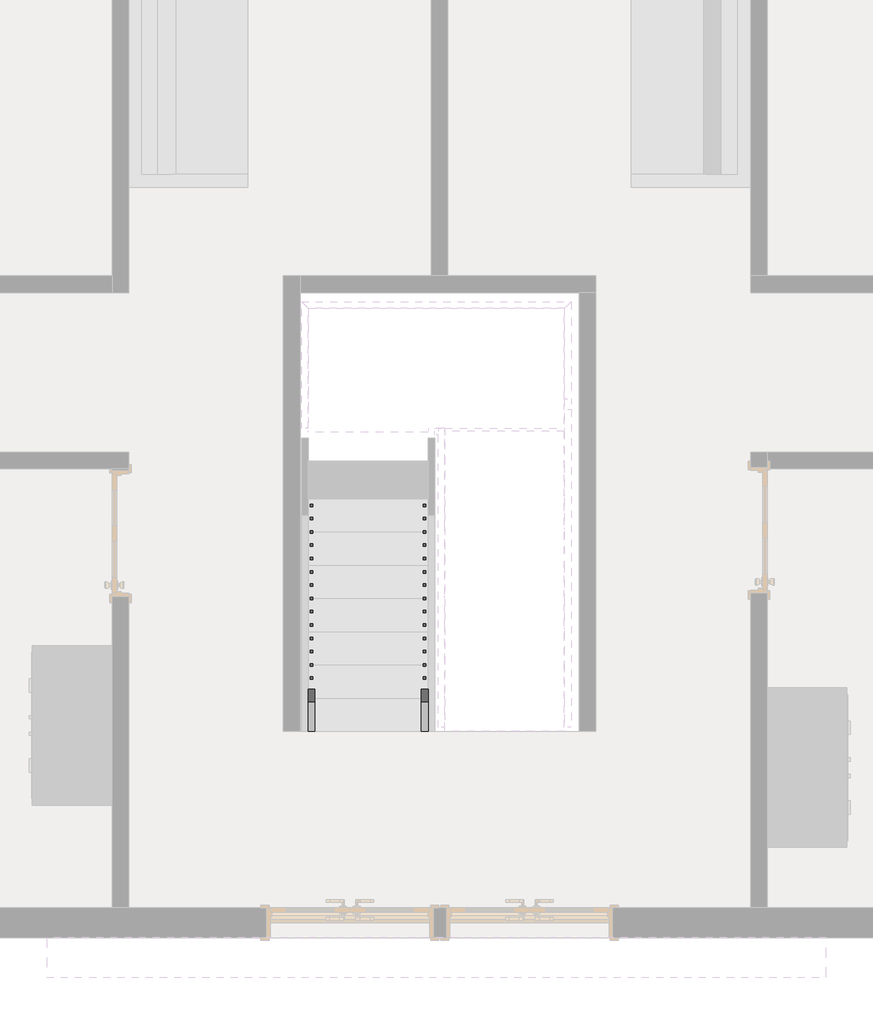
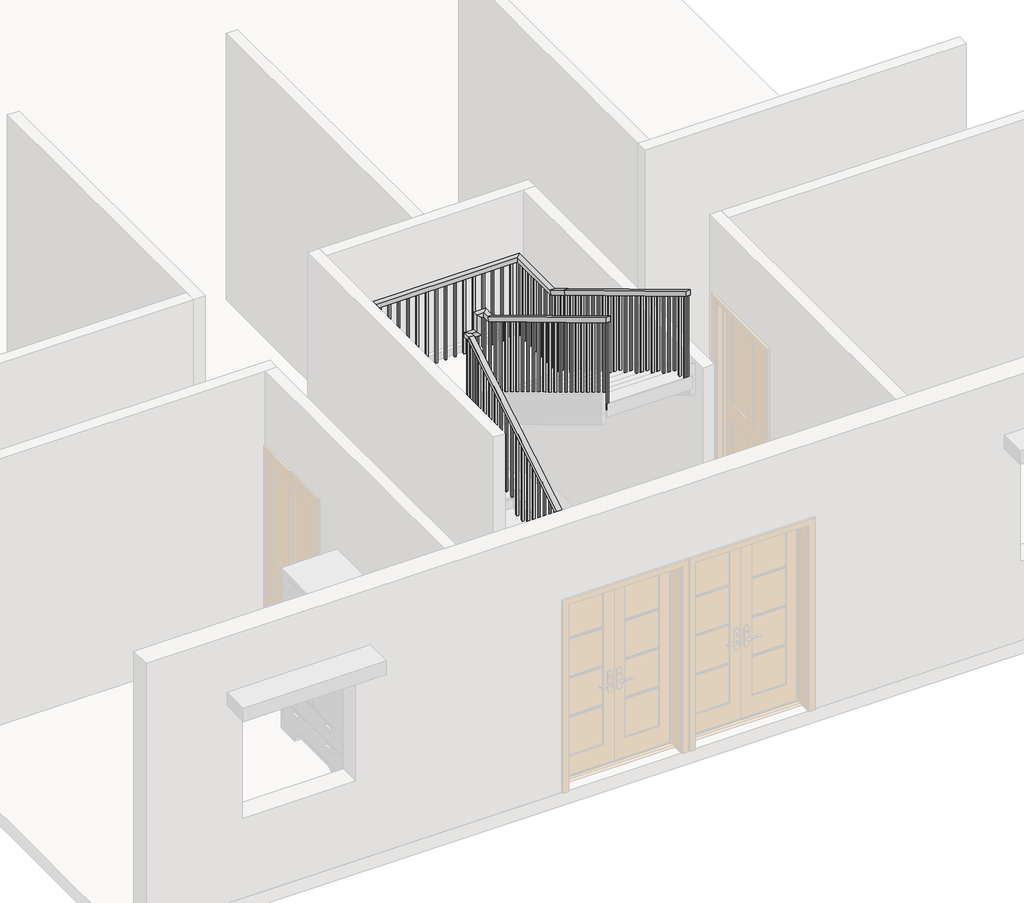
# One storey, part 3 of 4: 2 railings.
"""IFC4 building model written with IfcOpenShell, lengths in millimetres."""

from ifc_helpers import new_model, si_unit, frame, origin, place, context, project, spatial, polyline, outline, extrude, faceted_brep, element, save

model = new_model("IFC4")

# Units and contexts
model_context = context("Model", 3, world=origin())
ifc_project = project(units=[si_unit("LENGTHUNIT", "METRE", prefix="MILLI")], contexts=[model_context])

# Site, building, storey
site = spatial("IfcSite", under=ifc_project)
building = spatial("IfcBuilding", under=site)
storey = spatial("IfcBuildingStorey", under=building, Elevation=0.0)

# Railings
placement = place(None, origin())
element("IfcRailing", 1, ObjectType="Handrail - Rectangular", at=placement, inside=storey, context=model_context, shape_type="SolidModel", body=[
    faceted_brep([(-9678.6771954, -4957.4727897, 1066.8), (-9678.6771954, -4957.4727897, 1007.5575287), (-9627.8771954, -4957.4727897, 1007.5575287), (-9627.8771954, -4957.4727897, 1066.8), (-9678.6771954, -2671.4727897, 2438.4), (-9678.6771954, -2657.4020042, 2387.6), (-9627.8771954, -2657.4020042, 2387.6), (-9627.8771954, -2671.4727897, 2438.4), (-9678.6771954, -2588.9227897, 2438.4), (-9678.6771954, -2588.9227897, 2387.6), (-9627.8771954, -2639.7227897, 2387.6), (-9627.8771954, -2639.7227897, 2438.4), (-9577.0771954, -2588.9227897, 2438.4), (-9526.2771954, -2588.9227897, 2387.6), (-9526.2771954, -2639.7227897, 2387.6), (-9577.0771954, -2639.7227897, 2438.4), (-9577.0771954, -2588.9227897, 2636.52), (-9526.2771954, -2588.9227897, 2585.72), (-9526.2771954, -2639.7227897, 2585.72), (-9577.0771954, -2639.7227897, 2636.52), (-9450.0771954, -2588.9227897, 2636.52), (-9450.0771954, -2588.9227897, 2585.72), (-9500.8771954, -2639.7227897, 2585.72), (-9500.8771954, -2639.7227897, 2636.52), (-9450.0771954, -2715.9227897, 2636.52), (-9450.0771954, -2729.9935751, 2585.72), (-9500.8771954, -2729.9935751, 2585.72), (-9500.8771954, -2715.9227897, 2636.52), (-9450.0771954, -4925.7227897, 3962.4), (-9500.8771954, -4925.7227897, 3962.4), (-9500.8771954, -4925.7227897, 3903.1575287), (-9450.0771954, -4925.7227897, 3903.1575287)], [[[0, 1, 2, 3]], [[1, 0, 4, 5]], [[2, 1, 5, 6]], [[3, 2, 6, 7]], [[0, 3, 7, 4]], [[5, 4, 8, 9]], [[6, 5, 9, 10]], [[7, 6, 10, 11]], [[4, 7, 11, 8]], [[9, 8, 12, 13]], [[10, 9, 13, 14]], [[11, 10, 14, 15]], [[8, 11, 15, 12]], [[13, 12, 16, 17]], [[14, 13, 17, 18]], [[15, 14, 18, 19]], [[12, 15, 19, 16]], [[17, 16, 20, 21]], [[18, 17, 21, 22]], [[19, 18, 22, 23]], [[16, 19, 23, 20]], [[21, 20, 24, 25]], [[22, 21, 25, 26]], [[23, 22, 26, 27]], [[20, 23, 27, 24]], [[28, 29, 30, 31]], [[25, 24, 28, 31]], [[26, 25, 31, 30]], [[27, 26, 30, 29]], [[24, 27, 29, 28]]]),
    extrude(outline(polyline([(-4859.0477897, 3863.1525287), (-4839.9977897, 3851.7225287), (-4839.9977897, 2895.6), (-4859.0477897, 2895.6), (-4859.0477897, 3863.1525287)])), frame((-9485.0021954, 0.0, 0.0), z_axis=(1.0, 0.0, 0.0), x_axis=(0.0, 1.0, 0.0)), (0.0, 0.0, 1.0), 19.05),
    extrude(outline(polyline([(-4757.4477897, 3802.1925287), (-4738.3977897, 3790.7625287), (-4738.3977897, 2895.6), (-4757.4477897, 2895.6), (-4757.4477897, 3802.1925287)])), frame((-9485.0021954, 0.0, 0.0), z_axis=(1.0, 0.0, 0.0), x_axis=(0.0, 1.0, 0.0)), (0.0, 0.0, 1.0), 19.05),
    extrude(outline(polyline([(-4655.8477897, 3741.2325287), (-4636.7977897, 3729.8025287), (-4636.7977897, 2743.2), (-4655.8477897, 2743.2), (-4655.8477897, 3741.2325287)])), frame((-9485.0021954, 0.0, 0.0), z_axis=(1.0, 0.0, 0.0), x_axis=(0.0, 1.0, 0.0)), (0.0, 0.0, 1.0), 19.05),
    extrude(outline(polyline([(-4554.2477897, 3680.2725287), (-4535.1977897, 3668.8425287), (-4535.1977897, 2743.2), (-4554.2477897, 2743.2), (-4554.2477897, 3680.2725287)])), frame((-9485.0021954, 0.0, 0.0), z_axis=(1.0, 0.0, 0.0), x_axis=(0.0, 1.0, 0.0)), (0.0, 0.0, 1.0), 19.05),
    extrude(outline(polyline([(-4452.6477897, 3619.3125287), (-4433.5977897, 3607.8825287), (-4433.5977897, 2743.2), (-4452.6477897, 2743.2), (-4452.6477897, 3619.3125287)])), frame((-9485.0021954, 0.0, 0.0), z_axis=(1.0, 0.0, 0.0), x_axis=(0.0, 1.0, 0.0)), (0.0, 0.0, 1.0), 19.05),
    extrude(outline(polyline([(-4351.0477897, 3558.3525287), (-4331.9977897, 3546.9225287), (-4331.9977897, 2590.8), (-4351.0477897, 2590.8), (-4351.0477897, 3558.3525287)])), frame((-9485.0021954, 0.0, 0.0), z_axis=(1.0, 0.0, 0.0), x_axis=(0.0, 1.0, 0.0)), (0.0, 0.0, 1.0), 19.05),
    extrude(outline(polyline([(-4249.4477897, 3497.3925287), (-4230.3977897, 3485.9625287), (-4230.3977897, 2590.8), (-4249.4477897, 2590.8), (-4249.4477897, 3497.3925287)])), frame((-9485.0021954, 0.0, 0.0), z_axis=(1.0, 0.0, 0.0), x_axis=(0.0, 1.0, 0.0)), (0.0, 0.0, 1.0), 19.05),
    extrude(outline(polyline([(-4147.8477897, 3436.4325287), (-4128.7977897, 3425.0025287), (-4128.7977897, 2438.4), (-4147.8477897, 2438.4), (-4147.8477897, 3436.4325287)])), frame((-9485.0021954, 0.0, 0.0), z_axis=(1.0, 0.0, 0.0), x_axis=(0.0, 1.0, 0.0)), (0.0, 0.0, 1.0), 19.05),
    extrude(outline(polyline([(-4046.2477897, 3375.4725287), (-4027.1977897, 3364.0425287), (-4027.1977897, 2438.4), (-4046.2477897, 2438.4), (-4046.2477897, 3375.4725287)])), frame((-9485.0021954, 0.0, 0.0), z_axis=(1.0, 0.0, 0.0), x_axis=(0.0, 1.0, 0.0)), (0.0, 0.0, 1.0), 19.05),
    extrude(outline(polyline([(-3944.6477897, 3314.5125287), (-3925.5977897, 3303.0825287), (-3925.5977897, 2438.4), (-3944.6477897, 2438.4), (-3944.6477897, 3314.5125287)])), frame((-9485.0021954, 0.0, 0.0), z_axis=(1.0, 0.0, 0.0), x_axis=(0.0, 1.0, 0.0)), (0.0, 0.0, 1.0), 19.05),
    extrude(outline(polyline([(-3843.0477897, 3253.5525287), (-3823.9977897, 3242.1225287), (-3823.9977897, 2286.0), (-3843.0477897, 2286.0), (-3843.0477897, 3253.5525287)])), frame((-9485.0021954, 0.0, 0.0), z_axis=(1.0, 0.0, 0.0), x_axis=(0.0, 1.0, 0.0)), (0.0, 0.0, 1.0), 19.05),
    extrude(outline(polyline([(-3741.4477897, 3192.5925287), (-3722.3977897, 3181.1625287), (-3722.3977897, 2286.0), (-3741.4477897, 2286.0), (-3741.4477897, 3192.5925287)])), frame((-9485.0021954, 0.0, 0.0), z_axis=(1.0, 0.0, 0.0), x_axis=(0.0, 1.0, 0.0)), (0.0, 0.0, 1.0), 19.05),
    extrude(outline(polyline([(-3639.8477897, 3131.6325287), (-3620.7977897, 3120.2025287), (-3620.7977897, 2133.6), (-3639.8477897, 2133.6), (-3639.8477897, 3131.6325287)])), frame((-9485.0021954, 0.0, 0.0), z_axis=(1.0, 0.0, 0.0), x_axis=(0.0, 1.0, 0.0)), (0.0, 0.0, 1.0), 19.05),
    extrude(outline(polyline([(-3538.2477897, 3070.6725287), (-3519.1977897, 3059.2425287), (-3519.1977897, 2133.6), (-3538.2477897, 2133.6), (-3538.2477897, 3070.6725287)])), frame((-9485.0021954, 0.0, 0.0), z_axis=(1.0, 0.0, 0.0), x_axis=(0.0, 1.0, 0.0)), (0.0, 0.0, 1.0), 19.05),
    extrude(outline(polyline([(-3436.6477897, 3009.7125287), (-3417.5977897, 2998.2825287), (-3417.5977897, 2133.6), (-3436.6477897, 2133.6), (-3436.6477897, 3009.7125287)])), frame((-9485.0021954, 0.0, 0.0), z_axis=(1.0, 0.0, 0.0), x_axis=(0.0, 1.0, 0.0)), (0.0, 0.0, 1.0), 19.05),
    extrude(outline(polyline([(-3335.0477897, 2948.7525287), (-3315.9977897, 2937.3225287), (-3315.9977897, 1981.2), (-3335.0477897, 1981.2), (-3335.0477897, 2948.7525287)])), frame((-9485.0021954, 0.0, 0.0), z_axis=(1.0, 0.0, 0.0), x_axis=(0.0, 1.0, 0.0)), (0.0, 0.0, 1.0), 19.05),
    extrude(outline(polyline([(-3233.4477897, 2887.7925287), (-3214.3977897, 2876.3625287), (-3214.3977897, 1981.2), (-3233.4477897, 1981.2), (-3233.4477897, 2887.7925287)])), frame((-9485.0021954, 0.0, 0.0), z_axis=(1.0, 0.0, 0.0), x_axis=(0.0, 1.0, 0.0)), (0.0, 0.0, 1.0), 19.05),
    extrude(outline(polyline([(-3131.8477897, 2826.8325287), (-3112.7977897, 2815.4025287), (-3112.7977897, 1828.8), (-3131.8477897, 1828.8), (-3131.8477897, 2826.8325287)])), frame((-9485.0021954, 0.0, 0.0), z_axis=(1.0, 0.0, 0.0), x_axis=(0.0, 1.0, 0.0)), (0.0, 0.0, 1.0), 19.05),
    extrude(outline(polyline([(-3030.2477897, 2765.8725287), (-3011.1977897, 2754.4425287), (-3011.1977897, 1828.8), (-3030.2477897, 1828.8), (-3030.2477897, 2765.8725287)])), frame((-9485.0021954, 0.0, 0.0), z_axis=(1.0, 0.0, 0.0), x_axis=(0.0, 1.0, 0.0)), (0.0, 0.0, 1.0), 19.05),
    extrude(outline(polyline([(-2928.6477897, 2704.9125287), (-2909.5977897, 2693.4825287), (-2909.5977897, 1828.8), (-2928.6477897, 1828.8), (-2928.6477897, 2704.9125287)])), frame((-9485.0021954, 0.0, 0.0), z_axis=(1.0, 0.0, 0.0), x_axis=(0.0, 1.0, 0.0)), (0.0, 0.0, 1.0), 19.05),
    extrude(outline(polyline([(-2827.0477897, 2643.9525287), (-2807.9977897, 2632.5225287), (-2807.9977897, 1676.4), (-2827.0477897, 1676.4), (-2827.0477897, 2643.9525287)])), frame((-9485.0021954, 0.0, 0.0), z_axis=(1.0, 0.0, 0.0), x_axis=(0.0, 1.0, 0.0)), (0.0, 0.0, 1.0), 19.05),
    extrude(outline(polyline([(-2725.4477897, 2582.9925287), (-2706.3977897, 2571.5625287), (-2706.3977897, 1676.4), (-2725.4477897, 1676.4), (-2725.4477897, 2582.9925287)])), frame((-9485.0021954, 0.0, 0.0), z_axis=(1.0, 0.0, 0.0), x_axis=(0.0, 1.0, 0.0)), (0.0, 0.0, 1.0), 19.05),
    extrude(outline(polyline([(-9561.2021954, -2623.8477897), (-9561.2021954, -2604.7977897), (-9542.1521954, -2604.7977897), (-9542.1521954, -2623.8477897), (-9561.2021954, -2623.8477897)])), frame((0.0, 0.0, 1524.0), z_axis=(0.0, 0.0, 1.0), x_axis=(1.0, 0.0, 0.0)), (0.0, 0.0, 1.0), 1061.72),
    extrude(outline(polyline([(-2731.7977897, 2342.9625287), (-2712.7477897, 2354.3925287), (-2712.7477897, 1371.6), (-2731.7977897, 1371.6), (-2731.7977897, 2342.9625287)])), frame((-9662.8021954, 0.0, 0.0), z_axis=(1.0, 0.0, 0.0), x_axis=(0.0, 1.0, 0.0)), (0.0, 0.0, 1.0), 19.05),
    extrude(outline(polyline([(-2833.3977897, 2282.0025287), (-2814.3477897, 2293.4325287), (-2814.3477897, 1371.6), (-2833.3977897, 1371.6), (-2833.3977897, 2282.0025287)])), frame((-9662.8021954, 0.0, 0.0), z_axis=(1.0, 0.0, 0.0), x_axis=(0.0, 1.0, 0.0)), (0.0, 0.0, 1.0), 19.05),
    extrude(outline(polyline([(-2934.9977897, 2221.0425287), (-2915.9477897, 2232.4725287), (-2915.9477897, 1371.6), (-2934.9977897, 1371.6), (-2934.9977897, 2221.0425287)])), frame((-9662.8021954, 0.0, 0.0), z_axis=(1.0, 0.0, 0.0), x_axis=(0.0, 1.0, 0.0)), (0.0, 0.0, 1.0), 19.05),
    extrude(outline(polyline([(-3036.5977897, 2160.0825287), (-3017.5477897, 2171.5125287), (-3017.5477897, 1219.2), (-3036.5977897, 1219.2), (-3036.5977897, 2160.0825287)])), frame((-9662.8021954, 0.0, 0.0), z_axis=(1.0, 0.0, 0.0), x_axis=(0.0, 1.0, 0.0)), (0.0, 0.0, 1.0), 19.05),
    extrude(outline(polyline([(-3138.1977897, 2099.1225287), (-3119.1477897, 2110.5525287), (-3119.1477897, 1219.2), (-3138.1977897, 1219.2), (-3138.1977897, 2099.1225287)])), frame((-9662.8021954, 0.0, 0.0), z_axis=(1.0, 0.0, 0.0), x_axis=(0.0, 1.0, 0.0)), (0.0, 0.0, 1.0), 19.05),
    extrude(outline(polyline([(-3239.7977897, 2038.1625287), (-3220.7477897, 2049.5925287), (-3220.7477897, 1066.8), (-3239.7977897, 1066.8), (-3239.7977897, 2038.1625287)])), frame((-9662.8021954, 0.0, 0.0), z_axis=(1.0, 0.0, 0.0), x_axis=(0.0, 1.0, 0.0)), (0.0, 0.0, 1.0), 19.05),
    extrude(outline(polyline([(-3341.3977897, 1977.2025287), (-3322.3477897, 1988.6325287), (-3322.3477897, 1066.8), (-3341.3977897, 1066.8), (-3341.3977897, 1977.2025287)])), frame((-9662.8021954, 0.0, 0.0), z_axis=(1.0, 0.0, 0.0), x_axis=(0.0, 1.0, 0.0)), (0.0, 0.0, 1.0), 19.05),
    extrude(outline(polyline([(-3442.9977897, 1916.2425287), (-3423.9477897, 1927.6725287), (-3423.9477897, 1066.8), (-3442.9977897, 1066.8), (-3442.9977897, 1916.2425287)])), frame((-9662.8021954, 0.0, 0.0), z_axis=(1.0, 0.0, 0.0), x_axis=(0.0, 1.0, 0.0)), (0.0, 0.0, 1.0), 19.05),
    extrude(outline(polyline([(-3544.5977897, 1855.2825287), (-3525.5477897, 1866.7125287), (-3525.5477897, 914.4), (-3544.5977897, 914.4), (-3544.5977897, 1855.2825287)])), frame((-9662.8021954, 0.0, 0.0), z_axis=(1.0, 0.0, 0.0), x_axis=(0.0, 1.0, 0.0)), (0.0, 0.0, 1.0), 19.05),
    extrude(outline(polyline([(-3646.1977897, 1794.3225287), (-3627.1477897, 1805.7525287), (-3627.1477897, 914.4), (-3646.1977897, 914.4), (-3646.1977897, 1794.3225287)])), frame((-9662.8021954, 0.0, 0.0), z_axis=(1.0, 0.0, 0.0), x_axis=(0.0, 1.0, 0.0)), (0.0, 0.0, 1.0), 19.05),
    extrude(outline(polyline([(-3747.7977897, 1733.3625287), (-3728.7477897, 1744.7925287), (-3728.7477897, 762.0), (-3747.7977897, 762.0), (-3747.7977897, 1733.3625287)])), frame((-9662.8021954, 0.0, 0.0), z_axis=(1.0, 0.0, 0.0), x_axis=(0.0, 1.0, 0.0)), (0.0, 0.0, 1.0), 19.05),
    extrude(outline(polyline([(-3849.3977897, 1672.4025287), (-3830.3477897, 1683.8325287), (-3830.3477897, 762.0), (-3849.3977897, 762.0), (-3849.3977897, 1672.4025287)])), frame((-9662.8021954, 0.0, 0.0), z_axis=(1.0, 0.0, 0.0), x_axis=(0.0, 1.0, 0.0)), (0.0, 0.0, 1.0), 19.05),
    extrude(outline(polyline([(-3950.9977897, 1611.4425287), (-3931.9477897, 1622.8725287), (-3931.9477897, 762.0), (-3950.9977897, 762.0), (-3950.9977897, 1611.4425287)])), frame((-9662.8021954, 0.0, 0.0), z_axis=(1.0, 0.0, 0.0), x_axis=(0.0, 1.0, 0.0)), (0.0, 0.0, 1.0), 19.05),
    extrude(outline(polyline([(-4052.5977897, 1550.4825287), (-4033.5477897, 1561.9125287), (-4033.5477897, 609.6), (-4052.5977897, 609.6), (-4052.5977897, 1550.4825287)])), frame((-9662.8021954, 0.0, 0.0), z_axis=(1.0, 0.0, 0.0), x_axis=(0.0, 1.0, 0.0)), (0.0, 0.0, 1.0), 19.05),
    extrude(outline(polyline([(-4154.1977897, 1489.5225287), (-4135.1477897, 1500.9525287), (-4135.1477897, 609.6), (-4154.1977897, 609.6), (-4154.1977897, 1489.5225287)])), frame((-9662.8021954, 0.0, 0.0), z_axis=(1.0, 0.0, 0.0), x_axis=(0.0, 1.0, 0.0)), (0.0, 0.0, 1.0), 19.05),
    extrude(outline(polyline([(-4255.7977897, 1428.5625287), (-4236.7477897, 1439.9925287), (-4236.7477897, 457.2), (-4255.7977897, 457.2), (-4255.7977897, 1428.5625287)])), frame((-9662.8021954, 0.0, 0.0), z_axis=(1.0, 0.0, 0.0), x_axis=(0.0, 1.0, 0.0)), (0.0, 0.0, 1.0), 19.05),
    extrude(outline(polyline([(-4357.3977897, 1367.6025287), (-4338.3477897, 1379.0325287), (-4338.3477897, 457.2), (-4357.3977897, 457.2), (-4357.3977897, 1367.6025287)])), frame((-9662.8021954, 0.0, 0.0), z_axis=(1.0, 0.0, 0.0), x_axis=(0.0, 1.0, 0.0)), (0.0, 0.0, 1.0), 19.05),
    extrude(outline(polyline([(-4458.9977897, 1306.6425287), (-4439.9477897, 1318.0725287), (-4439.9477897, 457.2), (-4458.9977897, 457.2), (-4458.9977897, 1306.6425287)])), frame((-9662.8021954, 0.0, 0.0), z_axis=(1.0, 0.0, 0.0), x_axis=(0.0, 1.0, 0.0)), (0.0, 0.0, 1.0), 19.05),
    extrude(outline(polyline([(-4560.5977897, 1245.6825287), (-4541.5477897, 1257.1125287), (-4541.5477897, 304.8), (-4560.5977897, 304.8), (-4560.5977897, 1245.6825287)])), frame((-9662.8021954, 0.0, 0.0), z_axis=(1.0, 0.0, 0.0), x_axis=(0.0, 1.0, 0.0)), (0.0, 0.0, 1.0), 19.05),
    extrude(outline(polyline([(-4662.1977897, 1184.7225287), (-4643.1477897, 1196.1525287), (-4643.1477897, 304.8), (-4662.1977897, 304.8), (-4662.1977897, 1184.7225287)])), frame((-9662.8021954, 0.0, 0.0), z_axis=(1.0, 0.0, 0.0), x_axis=(0.0, 1.0, 0.0)), (0.0, 0.0, 1.0), 19.05),
    extrude(outline(polyline([(-4763.7977897, 1123.7625287), (-4744.7477897, 1135.1925287), (-4744.7477897, 152.4), (-4763.7977897, 152.4), (-4763.7977897, 1123.7625287)])), frame((-9662.8021954, 0.0, 0.0), z_axis=(1.0, 0.0, 0.0), x_axis=(0.0, 1.0, 0.0)), (0.0, 0.0, 1.0), 19.05),
    extrude(outline(polyline([(-4865.3977897, 1062.8025287), (-4846.3477897, 1074.2325287), (-4846.3477897, 152.4), (-4865.3977897, 152.4), (-4865.3977897, 1062.8025287)])), frame((-9662.8021954, 0.0, 0.0), z_axis=(1.0, 0.0, 0.0), x_axis=(0.0, 1.0, 0.0)), (0.0, 0.0, 1.0), 19.05),
    extrude(outline(polyline([(-9485.0021954, -2623.8477897), (-9485.0021954, -2604.7977897), (-9465.9521954, -2604.7977897), (-9465.9521954, -2623.8477897), (-9485.0021954, -2623.8477897)])), frame((0.0, 0.0, 1524.0), z_axis=(0.0, 0.0, 1.0), x_axis=(1.0, 0.0, 0.0)), (0.0, 0.0, 1.0), 1061.72),
    extrude(outline(polyline([(-9643.7521954, -2623.8477897), (-9662.8021954, -2623.8477897), (-9662.8021954, -2604.7977897), (-9643.7521954, -2604.7977897), (-9643.7521954, -2623.8477897)])), frame((0.0, 0.0, 1524.0), z_axis=(0.0, 0.0, 1.0), x_axis=(1.0, 0.0, 0.0)), (0.0, 0.0, 1.0), 863.6),
    extrude(outline(polyline([(-2680.9977897, 2373.4425287), (-2661.9477897, 2384.8725287), (-2661.9477897, 1524.0), (-2680.9977897, 1524.0), (-2680.9977897, 2373.4425287)])), frame((-9662.8021954, 0.0, 0.0), z_axis=(1.0, 0.0, 0.0), x_axis=(0.0, 1.0, 0.0)), (0.0, 0.0, 1.0), 19.05),
    extrude(outline(polyline([(-4925.7227897, 3903.1575287), (-4906.6727897, 3891.7275287), (-4906.6727897, 2895.6), (-4925.7227897, 2895.6), (-4925.7227897, 3903.1575287)])), frame((-9485.0021954, 0.0, 0.0), z_axis=(1.0, 0.0, 0.0), x_axis=(0.0, 1.0, 0.0)), (0.0, 0.0, 1.0), 19.05),
    extrude(outline(polyline([(-4957.4727897, 1007.5575287), (-4938.4227897, 1018.9875287), (-4938.4227897, 152.4), (-4957.4727897, 152.4), (-4957.4727897, 1007.5575287)])), frame((-9662.8021954, 0.0, 0.0), z_axis=(1.0, 0.0, 0.0), x_axis=(0.0, 1.0, 0.0)), (0.0, 0.0, 1.0), 19.05),
])
element("IfcRailing", 2, ObjectType="Handrail - Rectangular", at=placement, inside=storey, context=model_context, shape_type="SolidModel", body=[
    faceted_brep([(-10542.2771954, -4957.4727897, 1066.8), (-10542.2771954, -4957.4727897, 1007.5575287), (-10491.4771954, -4957.4727897, 1007.5575287), (-10491.4771954, -4957.4727897, 1066.8), (-10542.2771954, -2671.4727897, 2438.4), (-10542.2771954, -2657.4020042, 2387.6), (-10491.4771954, -2657.4020042, 2387.6), (-10491.4771954, -2671.4727897, 2438.4), (-10542.2771954, -1725.3227897, 2438.4), (-10542.2771954, -1725.3227897, 2387.6), (-10491.4771954, -1776.1227897, 2387.6), (-10491.4771954, -1776.1227897, 2438.4), (-8586.4771954, -1725.3227897, 2438.4), (-8586.4771954, -1725.3227897, 2387.6), (-8637.2771954, -1776.1227897, 2387.6), (-8637.2771954, -1776.1227897, 2438.4), (-8586.4771954, -2385.7227897, 2438.4), (-8586.4771954, -2399.7935751, 2387.6), (-8637.2771954, -2399.7935751, 2387.6), (-8637.2771954, -2385.7227897, 2438.4), (-8586.4771954, -2639.7227897, 2590.8), (-8586.4771954, -2665.859174, 2547.2393594), (-8637.2771954, -2665.859174, 2547.2393594), (-8637.2771954, -2639.7227897, 2590.8), (-8586.4771954, -4925.7227897, 3962.4), (-8637.2771954, -4925.7227897, 3962.4), (-8637.2771954, -4925.7227897, 3903.1575287), (-8586.4771954, -4925.7227897, 3903.1575287)], [[[0, 1, 2, 3]], [[1, 0, 4, 5]], [[2, 1, 5, 6]], [[3, 2, 6, 7]], [[0, 3, 7, 4]], [[5, 4, 8, 9]], [[6, 5, 9, 10]], [[7, 6, 10, 11]], [[4, 7, 11, 8]], [[9, 8, 12, 13]], [[10, 9, 13, 14]], [[11, 10, 14, 15]], [[8, 11, 15, 12]], [[13, 12, 16, 17]], [[14, 13, 17, 18]], [[15, 14, 18, 19]], [[12, 15, 19, 16]], [[17, 16, 20, 21]], [[18, 17, 21, 22]], [[19, 18, 22, 23]], [[16, 19, 23, 20]], [[24, 25, 26, 27]], [[21, 20, 24, 27]], [[22, 21, 27, 26]], [[23, 22, 26, 25]], [[20, 23, 25, 24]]]),
    extrude(outline(polyline([(-4865.3977897, 3866.9625287), (-4865.3977897, 2895.6), (-4884.4477897, 2895.6), (-4884.4477897, 3878.3925287), (-4865.3977897, 3866.9625287)])), frame((-8621.4021954, 0.0, 0.0), z_axis=(1.0, 0.0, 0.0), x_axis=(0.0, 1.0, 0.0)), (0.0, 0.0, 1.0), 19.05),
    extrude(outline(polyline([(-4763.7977897, 3806.0025287), (-4763.7977897, 2895.6), (-4782.8477897, 2895.6), (-4782.8477897, 3817.4325287), (-4763.7977897, 3806.0025287)])), frame((-8621.4021954, 0.0, 0.0), z_axis=(1.0, 0.0, 0.0), x_axis=(0.0, 1.0, 0.0)), (0.0, 0.0, 1.0), 19.05),
    extrude(outline(polyline([(-4662.1977897, 3745.0425287), (-4662.1977897, 2895.6), (-4681.2477897, 2895.6), (-4681.2477897, 3756.4725287), (-4662.1977897, 3745.0425287)])), frame((-8621.4021954, 0.0, 0.0), z_axis=(1.0, 0.0, 0.0), x_axis=(0.0, 1.0, 0.0)), (0.0, 0.0, 1.0), 19.05),
    extrude(outline(polyline([(-4560.5977897, 3684.0825287), (-4560.5977897, 2743.2), (-4579.6477897, 2743.2), (-4579.6477897, 3695.5125287), (-4560.5977897, 3684.0825287)])), frame((-8621.4021954, 0.0, 0.0), z_axis=(1.0, 0.0, 0.0), x_axis=(0.0, 1.0, 0.0)), (0.0, 0.0, 1.0), 19.05),
    extrude(outline(polyline([(-4458.9977897, 3623.1225287), (-4458.9977897, 2743.2), (-4478.0477897, 2743.2), (-4478.0477897, 3634.5525287), (-4458.9977897, 3623.1225287)])), frame((-8621.4021954, 0.0, 0.0), z_axis=(1.0, 0.0, 0.0), x_axis=(0.0, 1.0, 0.0)), (0.0, 0.0, 1.0), 19.05),
    extrude(outline(polyline([(-4357.3977897, 3562.1625287), (-4357.3977897, 2590.8), (-4376.4477897, 2590.8), (-4376.4477897, 3573.5925287), (-4357.3977897, 3562.1625287)])), frame((-8621.4021954, 0.0, 0.0), z_axis=(1.0, 0.0, 0.0), x_axis=(0.0, 1.0, 0.0)), (0.0, 0.0, 1.0), 19.05),
    extrude(outline(polyline([(-4255.7977897, 3501.2025287), (-4255.7977897, 2590.8), (-4274.8477897, 2590.8), (-4274.8477897, 3512.6325287), (-4255.7977897, 3501.2025287)])), frame((-8621.4021954, 0.0, 0.0), z_axis=(1.0, 0.0, 0.0), x_axis=(0.0, 1.0, 0.0)), (0.0, 0.0, 1.0), 19.05),
    extrude(outline(polyline([(-4154.1977897, 3440.2425287), (-4154.1977897, 2590.8), (-4173.2477897, 2590.8), (-4173.2477897, 3451.6725287), (-4154.1977897, 3440.2425287)])), frame((-8621.4021954, 0.0, 0.0), z_axis=(1.0, 0.0, 0.0), x_axis=(0.0, 1.0, 0.0)), (0.0, 0.0, 1.0), 19.05),
    extrude(outline(polyline([(-4052.5977897, 3379.2825287), (-4052.5977897, 2438.4), (-4071.6477897, 2438.4), (-4071.6477897, 3390.7125287), (-4052.5977897, 3379.2825287)])), frame((-8621.4021954, 0.0, 0.0), z_axis=(1.0, 0.0, 0.0), x_axis=(0.0, 1.0, 0.0)), (0.0, 0.0, 1.0), 19.05),
    extrude(outline(polyline([(-3950.9977897, 3318.3225287), (-3950.9977897, 2438.4), (-3970.0477897, 2438.4), (-3970.0477897, 3329.7525287), (-3950.9977897, 3318.3225287)])), frame((-8621.4021954, 0.0, 0.0), z_axis=(1.0, 0.0, 0.0), x_axis=(0.0, 1.0, 0.0)), (0.0, 0.0, 1.0), 19.05),
    extrude(outline(polyline([(-3849.3977897, 3257.3625287), (-3849.3977897, 2286.0), (-3868.4477897, 2286.0), (-3868.4477897, 3268.7925287), (-3849.3977897, 3257.3625287)])), frame((-8621.4021954, 0.0, 0.0), z_axis=(1.0, 0.0, 0.0), x_axis=(0.0, 1.0, 0.0)), (0.0, 0.0, 1.0), 19.05),
    extrude(outline(polyline([(-3747.7977897, 3196.4025287), (-3747.7977897, 2286.0), (-3766.8477897, 2286.0), (-3766.8477897, 3207.8325287), (-3747.7977897, 3196.4025287)])), frame((-8621.4021954, 0.0, 0.0), z_axis=(1.0, 0.0, 0.0), x_axis=(0.0, 1.0, 0.0)), (0.0, 0.0, 1.0), 19.05),
    extrude(outline(polyline([(-3646.1977897, 3135.4425287), (-3646.1977897, 2286.0), (-3665.2477897, 2286.0), (-3665.2477897, 3146.8725287), (-3646.1977897, 3135.4425287)])), frame((-8621.4021954, 0.0, 0.0), z_axis=(1.0, 0.0, 0.0), x_axis=(0.0, 1.0, 0.0)), (0.0, 0.0, 1.0), 19.05),
    extrude(outline(polyline([(-3544.5977897, 3074.4825287), (-3544.5977897, 2133.6), (-3563.6477897, 2133.6), (-3563.6477897, 3085.9125287), (-3544.5977897, 3074.4825287)])), frame((-8621.4021954, 0.0, 0.0), z_axis=(1.0, 0.0, 0.0), x_axis=(0.0, 1.0, 0.0)), (0.0, 0.0, 1.0), 19.05),
    extrude(outline(polyline([(-3442.9977897, 3013.5225287), (-3442.9977897, 2133.6), (-3462.0477897, 2133.6), (-3462.0477897, 3024.9525287), (-3442.9977897, 3013.5225287)])), frame((-8621.4021954, 0.0, 0.0), z_axis=(1.0, 0.0, 0.0), x_axis=(0.0, 1.0, 0.0)), (0.0, 0.0, 1.0), 19.05),
    extrude(outline(polyline([(-3341.3977897, 2952.5625287), (-3341.3977897, 1981.2), (-3360.4477897, 1981.2), (-3360.4477897, 2963.9925287), (-3341.3977897, 2952.5625287)])), frame((-8621.4021954, 0.0, 0.0), z_axis=(1.0, 0.0, 0.0), x_axis=(0.0, 1.0, 0.0)), (0.0, 0.0, 1.0), 19.05),
    extrude(outline(polyline([(-3239.7977897, 2891.6025287), (-3239.7977897, 1981.2), (-3258.8477897, 1981.2), (-3258.8477897, 2903.0325287), (-3239.7977897, 2891.6025287)])), frame((-8621.4021954, 0.0, 0.0), z_axis=(1.0, 0.0, 0.0), x_axis=(0.0, 1.0, 0.0)), (0.0, 0.0, 1.0), 19.05),
    extrude(outline(polyline([(-3138.1977897, 2830.6425287), (-3138.1977897, 1981.2), (-3157.2477897, 1981.2), (-3157.2477897, 2842.0725287), (-3138.1977897, 2830.6425287)])), frame((-8621.4021954, 0.0, 0.0), z_axis=(1.0, 0.0, 0.0), x_axis=(0.0, 1.0, 0.0)), (0.0, 0.0, 1.0), 19.05),
    extrude(outline(polyline([(-3036.5977897, 2769.6825287), (-3036.5977897, 1828.8), (-3055.6477897, 1828.8), (-3055.6477897, 2781.1125287), (-3036.5977897, 2769.6825287)])), frame((-8621.4021954, 0.0, 0.0), z_axis=(1.0, 0.0, 0.0), x_axis=(0.0, 1.0, 0.0)), (0.0, 0.0, 1.0), 19.05),
    extrude(outline(polyline([(-2934.9977897, 2708.7225287), (-2934.9977897, 1828.8), (-2954.0477897, 1828.8), (-2954.0477897, 2720.1525287), (-2934.9977897, 2708.7225287)])), frame((-8621.4021954, 0.0, 0.0), z_axis=(1.0, 0.0, 0.0), x_axis=(0.0, 1.0, 0.0)), (0.0, 0.0, 1.0), 19.05),
    extrude(outline(polyline([(-2833.3977897, 2647.7625287), (-2833.3977897, 1676.4), (-2852.4477897, 1676.4), (-2852.4477897, 2659.1925287), (-2833.3977897, 2647.7625287)])), frame((-8621.4021954, 0.0, 0.0), z_axis=(1.0, 0.0, 0.0), x_axis=(0.0, 1.0, 0.0)), (0.0, 0.0, 1.0), 19.05),
    extrude(outline(polyline([(-2731.7977897, 2586.8025287), (-2731.7977897, 1676.4), (-2750.8477897, 1676.4), (-2750.8477897, 2598.2325287), (-2731.7977897, 2586.8025287)])), frame((-8621.4021954, 0.0, 0.0), z_axis=(1.0, 0.0, 0.0), x_axis=(0.0, 1.0, 0.0)), (0.0, 0.0, 1.0), 19.05),
    extrude(outline(polyline([(-2553.9977897, 2480.1225287), (-2553.9977897, 1524.0), (-2573.0477897, 1524.0), (-2573.0477897, 2491.5525287), (-2553.9977897, 2480.1225287)])), frame((-8621.4021954, 0.0, 0.0), z_axis=(1.0, 0.0, 0.0), x_axis=(0.0, 1.0, 0.0)), (0.0, 0.0, 1.0), 19.05),
    extrude(outline(polyline([(-2452.3977897, 2419.1625287), (-2452.3977897, 1524.0), (-2471.4477897, 1524.0), (-2471.4477897, 2430.5925287), (-2452.3977897, 2419.1625287)])), frame((-8621.4021954, 0.0, 0.0), z_axis=(1.0, 0.0, 0.0), x_axis=(0.0, 1.0, 0.0)), (0.0, 0.0, 1.0), 19.05),
    extrude(outline(polyline([(-8602.3521954, -2350.7977897), (-8602.3521954, -2369.8477897), (-8621.4021954, -2369.8477897), (-8621.4021954, -2350.7977897), (-8602.3521954, -2350.7977897)])), frame((0.0, 0.0, 1524.0), z_axis=(0.0, 0.0, 1.0), x_axis=(1.0, 0.0, 0.0)), (0.0, 0.0, 1.0), 863.6),
    extrude(outline(polyline([(-8602.3521954, -2249.1977897), (-8602.3521954, -2268.2477897), (-8621.4021954, -2268.2477897), (-8621.4021954, -2249.1977897), (-8602.3521954, -2249.1977897)])), frame((0.0, 0.0, 1524.0), z_axis=(0.0, 0.0, 1.0), x_axis=(1.0, 0.0, 0.0)), (0.0, 0.0, 1.0), 863.6),
    extrude(outline(polyline([(-8602.3521954, -2147.5977897), (-8602.3521954, -2166.6477897), (-8621.4021954, -2166.6477897), (-8621.4021954, -2147.5977897), (-8602.3521954, -2147.5977897)])), frame((0.0, 0.0, 1524.0), z_axis=(0.0, 0.0, 1.0), x_axis=(1.0, 0.0, 0.0)), (0.0, 0.0, 1.0), 863.6),
    extrude(outline(polyline([(-8602.3521954, -2045.9977897), (-8602.3521954, -2065.0477897), (-8621.4021954, -2065.0477897), (-8621.4021954, -2045.9977897), (-8602.3521954, -2045.9977897)])), frame((0.0, 0.0, 1524.0), z_axis=(0.0, 0.0, 1.0), x_axis=(1.0, 0.0, 0.0)), (0.0, 0.0, 1.0), 863.6),
    extrude(outline(polyline([(-8602.3521954, -1944.3977897), (-8602.3521954, -1963.4477897), (-8621.4021954, -1963.4477897), (-8621.4021954, -1944.3977897), (-8602.3521954, -1944.3977897)])), frame((0.0, 0.0, 1524.0), z_axis=(0.0, 0.0, 1.0), x_axis=(1.0, 0.0, 0.0)), (0.0, 0.0, 1.0), 863.6),
    extrude(outline(polyline([(-8602.3521954, -1842.7977897), (-8602.3521954, -1861.8477897), (-8621.4021954, -1861.8477897), (-8621.4021954, -1842.7977897), (-8602.3521954, -1842.7977897)])), frame((0.0, 0.0, 1524.0), z_axis=(0.0, 0.0, 1.0), x_axis=(1.0, 0.0, 0.0)), (0.0, 0.0, 1.0), 863.6),
    extrude(outline(polyline([(-8697.6021954, -1741.1977897), (-8678.5521954, -1741.1977897), (-8678.5521954, -1760.2477897), (-8697.6021954, -1760.2477897), (-8697.6021954, -1741.1977897)])), frame((0.0, 0.0, 1524.0), z_axis=(0.0, 0.0, 1.0), x_axis=(1.0, 0.0, 0.0)), (0.0, 0.0, 1.0), 863.6),
    extrude(outline(polyline([(-8799.2021954, -1741.1977897), (-8780.1521954, -1741.1977897), (-8780.1521954, -1760.2477897), (-8799.2021954, -1760.2477897), (-8799.2021954, -1741.1977897)])), frame((0.0, 0.0, 1524.0), z_axis=(0.0, 0.0, 1.0), x_axis=(1.0, 0.0, 0.0)), (0.0, 0.0, 1.0), 863.6),
    extrude(outline(polyline([(-8900.8021954, -1741.1977897), (-8881.7521954, -1741.1977897), (-8881.7521954, -1760.2477897), (-8900.8021954, -1760.2477897), (-8900.8021954, -1741.1977897)])), frame((0.0, 0.0, 1524.0), z_axis=(0.0, 0.0, 1.0), x_axis=(1.0, 0.0, 0.0)), (0.0, 0.0, 1.0), 863.6),
    extrude(outline(polyline([(-9002.4021954, -1741.1977897), (-8983.3521954, -1741.1977897), (-8983.3521954, -1760.2477897), (-9002.4021954, -1760.2477897), (-9002.4021954, -1741.1977897)])), frame((0.0, 0.0, 1524.0), z_axis=(0.0, 0.0, 1.0), x_axis=(1.0, 0.0, 0.0)), (0.0, 0.0, 1.0), 863.6),
    extrude(outline(polyline([(-9104.0021954, -1741.1977897), (-9084.9521954, -1741.1977897), (-9084.9521954, -1760.2477897), (-9104.0021954, -1760.2477897), (-9104.0021954, -1741.1977897)])), frame((0.0, 0.0, 1524.0), z_axis=(0.0, 0.0, 1.0), x_axis=(1.0, 0.0, 0.0)), (0.0, 0.0, 1.0), 863.6),
    extrude(outline(polyline([(-9205.6021954, -1741.1977897), (-9186.5521954, -1741.1977897), (-9186.5521954, -1760.2477897), (-9205.6021954, -1760.2477897), (-9205.6021954, -1741.1977897)])), frame((0.0, 0.0, 1524.0), z_axis=(0.0, 0.0, 1.0), x_axis=(1.0, 0.0, 0.0)), (0.0, 0.0, 1.0), 863.6),
    extrude(outline(polyline([(-9307.2021954, -1741.1977897), (-9288.1521954, -1741.1977897), (-9288.1521954, -1760.2477897), (-9307.2021954, -1760.2477897), (-9307.2021954, -1741.1977897)])), frame((0.0, 0.0, 1524.0), z_axis=(0.0, 0.0, 1.0), x_axis=(1.0, 0.0, 0.0)), (0.0, 0.0, 1.0), 863.6),
    extrude(outline(polyline([(-9408.8021954, -1741.1977897), (-9389.7521954, -1741.1977897), (-9389.7521954, -1760.2477897), (-9408.8021954, -1760.2477897), (-9408.8021954, -1741.1977897)])), frame((0.0, 0.0, 1524.0), z_axis=(0.0, 0.0, 1.0), x_axis=(1.0, 0.0, 0.0)), (0.0, 0.0, 1.0), 863.6),
    extrude(outline(polyline([(-9510.4021954, -1741.1977897), (-9491.3521954, -1741.1977897), (-9491.3521954, -1760.2477897), (-9510.4021954, -1760.2477897), (-9510.4021954, -1741.1977897)])), frame((0.0, 0.0, 1524.0), z_axis=(0.0, 0.0, 1.0), x_axis=(1.0, 0.0, 0.0)), (0.0, 0.0, 1.0), 863.6),
    extrude(outline(polyline([(-9612.0021954, -1741.1977897), (-9592.9521954, -1741.1977897), (-9592.9521954, -1760.2477897), (-9612.0021954, -1760.2477897), (-9612.0021954, -1741.1977897)])), frame((0.0, 0.0, 1524.0), z_axis=(0.0, 0.0, 1.0), x_axis=(1.0, 0.0, 0.0)), (0.0, 0.0, 1.0), 863.6),
    extrude(outline(polyline([(-9713.6021954, -1741.1977897), (-9694.5521954, -1741.1977897), (-9694.5521954, -1760.2477897), (-9713.6021954, -1760.2477897), (-9713.6021954, -1741.1977897)])), frame((0.0, 0.0, 1524.0), z_axis=(0.0, 0.0, 1.0), x_axis=(1.0, 0.0, 0.0)), (0.0, 0.0, 1.0), 863.6),
    extrude(outline(polyline([(-9815.2021954, -1741.1977897), (-9796.1521954, -1741.1977897), (-9796.1521954, -1760.2477897), (-9815.2021954, -1760.2477897), (-9815.2021954, -1741.1977897)])), frame((0.0, 0.0, 1524.0), z_axis=(0.0, 0.0, 1.0), x_axis=(1.0, 0.0, 0.0)), (0.0, 0.0, 1.0), 863.6),
    extrude(outline(polyline([(-9916.8021954, -1741.1977897), (-9897.7521954, -1741.1977897), (-9897.7521954, -1760.2477897), (-9916.8021954, -1760.2477897), (-9916.8021954, -1741.1977897)])), frame((0.0, 0.0, 1524.0), z_axis=(0.0, 0.0, 1.0), x_axis=(1.0, 0.0, 0.0)), (0.0, 0.0, 1.0), 863.6),
    extrude(outline(polyline([(-10018.4021954, -1741.1977897), (-9999.3521954, -1741.1977897), (-9999.3521954, -1760.2477897), (-10018.4021954, -1760.2477897), (-10018.4021954, -1741.1977897)])), frame((0.0, 0.0, 1524.0), z_axis=(0.0, 0.0, 1.0), x_axis=(1.0, 0.0, 0.0)), (0.0, 0.0, 1.0), 863.6),
    extrude(outline(polyline([(-10120.0021954, -1741.1977897), (-10100.9521954, -1741.1977897), (-10100.9521954, -1760.2477897), (-10120.0021954, -1760.2477897), (-10120.0021954, -1741.1977897)])), frame((0.0, 0.0, 1524.0), z_axis=(0.0, 0.0, 1.0), x_axis=(1.0, 0.0, 0.0)), (0.0, 0.0, 1.0), 863.6),
    extrude(outline(polyline([(-10221.6021954, -1741.1977897), (-10202.5521954, -1741.1977897), (-10202.5521954, -1760.2477897), (-10221.6021954, -1760.2477897), (-10221.6021954, -1741.1977897)])), frame((0.0, 0.0, 1524.0), z_axis=(0.0, 0.0, 1.0), x_axis=(1.0, 0.0, 0.0)), (0.0, 0.0, 1.0), 863.6),
    extrude(outline(polyline([(-10323.2021954, -1741.1977897), (-10304.1521954, -1741.1977897), (-10304.1521954, -1760.2477897), (-10323.2021954, -1760.2477897), (-10323.2021954, -1741.1977897)])), frame((0.0, 0.0, 1524.0), z_axis=(0.0, 0.0, 1.0), x_axis=(1.0, 0.0, 0.0)), (0.0, 0.0, 1.0), 863.6),
    extrude(outline(polyline([(-10424.8021954, -1741.1977897), (-10405.7521954, -1741.1977897), (-10405.7521954, -1760.2477897), (-10424.8021954, -1760.2477897), (-10424.8021954, -1741.1977897)])), frame((0.0, 0.0, 1524.0), z_axis=(0.0, 0.0, 1.0), x_axis=(1.0, 0.0, 0.0)), (0.0, 0.0, 1.0), 863.6),
    extrude(outline(polyline([(-10526.4021954, -1766.5977897), (-10526.4021954, -1747.5477897), (-10507.3521954, -1747.5477897), (-10507.3521954, -1766.5977897), (-10526.4021954, -1766.5977897)])), frame((0.0, 0.0, 1524.0), z_axis=(0.0, 0.0, 1.0), x_axis=(1.0, 0.0, 0.0)), (0.0, 0.0, 1.0), 863.6),
    extrude(outline(polyline([(-10526.4021954, -1868.1977897), (-10526.4021954, -1849.1477897), (-10507.3521954, -1849.1477897), (-10507.3521954, -1868.1977897), (-10526.4021954, -1868.1977897)])), frame((0.0, 0.0, 1524.0), z_axis=(0.0, 0.0, 1.0), x_axis=(1.0, 0.0, 0.0)), (0.0, 0.0, 1.0), 863.6),
    extrude(outline(polyline([(-10526.4021954, -1969.7977897), (-10526.4021954, -1950.7477897), (-10507.3521954, -1950.7477897), (-10507.3521954, -1969.7977897), (-10526.4021954, -1969.7977897)])), frame((0.0, 0.0, 1524.0), z_axis=(0.0, 0.0, 1.0), x_axis=(1.0, 0.0, 0.0)), (0.0, 0.0, 1.0), 863.6),
    extrude(outline(polyline([(-10526.4021954, -2071.3977897), (-10526.4021954, -2052.3477897), (-10507.3521954, -2052.3477897), (-10507.3521954, -2071.3977897), (-10526.4021954, -2071.3977897)])), frame((0.0, 0.0, 1524.0), z_axis=(0.0, 0.0, 1.0), x_axis=(1.0, 0.0, 0.0)), (0.0, 0.0, 1.0), 863.6),
    extrude(outline(polyline([(-10526.4021954, -2172.9977897), (-10526.4021954, -2153.9477897), (-10507.3521954, -2153.9477897), (-10507.3521954, -2172.9977897), (-10526.4021954, -2172.9977897)])), frame((0.0, 0.0, 1524.0), z_axis=(0.0, 0.0, 1.0), x_axis=(1.0, 0.0, 0.0)), (0.0, 0.0, 1.0), 863.6),
    extrude(outline(polyline([(-10526.4021954, -2274.5977897), (-10526.4021954, -2255.5477897), (-10507.3521954, -2255.5477897), (-10507.3521954, -2274.5977897), (-10526.4021954, -2274.5977897)])), frame((0.0, 0.0, 1524.0), z_axis=(0.0, 0.0, 1.0), x_axis=(1.0, 0.0, 0.0)), (0.0, 0.0, 1.0), 863.6),
    extrude(outline(polyline([(-10526.4021954, -2376.1977897), (-10526.4021954, -2357.1477897), (-10507.3521954, -2357.1477897), (-10507.3521954, -2376.1977897), (-10526.4021954, -2376.1977897)])), frame((0.0, 0.0, 1524.0), z_axis=(0.0, 0.0, 1.0), x_axis=(1.0, 0.0, 0.0)), (0.0, 0.0, 1.0), 863.6),
    extrude(outline(polyline([(-10526.4021954, -2477.7977897), (-10526.4021954, -2458.7477897), (-10507.3521954, -2458.7477897), (-10507.3521954, -2477.7977897), (-10526.4021954, -2477.7977897)])), frame((0.0, 0.0, 1524.0), z_axis=(0.0, 0.0, 1.0), x_axis=(1.0, 0.0, 0.0)), (0.0, 0.0, 1.0), 863.6),
    extrude(outline(polyline([(-10526.4021954, -2579.3977897), (-10526.4021954, -2560.3477897), (-10507.3521954, -2560.3477897), (-10507.3521954, -2579.3977897), (-10526.4021954, -2579.3977897)])), frame((0.0, 0.0, 1524.0), z_axis=(0.0, 0.0, 1.0), x_axis=(1.0, 0.0, 0.0)), (0.0, 0.0, 1.0), 863.6),
    extrude(outline(polyline([(-2712.7477897, 2354.3925287), (-2712.7477897, 1371.6), (-2731.7977897, 1371.6), (-2731.7977897, 2342.9625287), (-2712.7477897, 2354.3925287)])), frame((-10526.4021954, 0.0, 0.0), z_axis=(1.0, 0.0, 0.0), x_axis=(0.0, 1.0, 0.0)), (0.0, 0.0, 1.0), 19.05),
    extrude(outline(polyline([(-2814.3477897, 2293.4325287), (-2814.3477897, 1371.6), (-2833.3977897, 1371.6), (-2833.3977897, 2282.0025287), (-2814.3477897, 2293.4325287)])), frame((-10526.4021954, 0.0, 0.0), z_axis=(1.0, 0.0, 0.0), x_axis=(0.0, 1.0, 0.0)), (0.0, 0.0, 1.0), 19.05),
    extrude(outline(polyline([(-2915.9477897, 2232.4725287), (-2915.9477897, 1371.6), (-2934.9977897, 1371.6), (-2934.9977897, 2221.0425287), (-2915.9477897, 2232.4725287)])), frame((-10526.4021954, 0.0, 0.0), z_axis=(1.0, 0.0, 0.0), x_axis=(0.0, 1.0, 0.0)), (0.0, 0.0, 1.0), 19.05),
    extrude(outline(polyline([(-3017.5477897, 2171.5125287), (-3017.5477897, 1219.2), (-3036.5977897, 1219.2), (-3036.5977897, 2160.0825287), (-3017.5477897, 2171.5125287)])), frame((-10526.4021954, 0.0, 0.0), z_axis=(1.0, 0.0, 0.0), x_axis=(0.0, 1.0, 0.0)), (0.0, 0.0, 1.0), 19.05),
    extrude(outline(polyline([(-3119.1477897, 2110.5525287), (-3119.1477897, 1219.2), (-3138.1977897, 1219.2), (-3138.1977897, 2099.1225287), (-3119.1477897, 2110.5525287)])), frame((-10526.4021954, 0.0, 0.0), z_axis=(1.0, 0.0, 0.0), x_axis=(0.0, 1.0, 0.0)), (0.0, 0.0, 1.0), 19.05),
    extrude(outline(polyline([(-3220.7477897, 2049.5925287), (-3220.7477897, 1066.8), (-3239.7977897, 1066.8), (-3239.7977897, 2038.1625287), (-3220.7477897, 2049.5925287)])), frame((-10526.4021954, 0.0, 0.0), z_axis=(1.0, 0.0, 0.0), x_axis=(0.0, 1.0, 0.0)), (0.0, 0.0, 1.0), 19.05),
    extrude(outline(polyline([(-3322.3477897, 1988.6325287), (-3322.3477897, 1066.8), (-3341.3977897, 1066.8), (-3341.3977897, 1977.2025287), (-3322.3477897, 1988.6325287)])), frame((-10526.4021954, 0.0, 0.0), z_axis=(1.0, 0.0, 0.0), x_axis=(0.0, 1.0, 0.0)), (0.0, 0.0, 1.0), 19.05),
    extrude(outline(polyline([(-3423.9477897, 1927.6725287), (-3423.9477897, 1066.8), (-3442.9977897, 1066.8), (-3442.9977897, 1916.2425287), (-3423.9477897, 1927.6725287)])), frame((-10526.4021954, 0.0, 0.0), z_axis=(1.0, 0.0, 0.0), x_axis=(0.0, 1.0, 0.0)), (0.0, 0.0, 1.0), 19.05),
    extrude(outline(polyline([(-3525.5477897, 1866.7125287), (-3525.5477897, 914.4), (-3544.5977897, 914.4), (-3544.5977897, 1855.2825287), (-3525.5477897, 1866.7125287)])), frame((-10526.4021954, 0.0, 0.0), z_axis=(1.0, 0.0, 0.0), x_axis=(0.0, 1.0, 0.0)), (0.0, 0.0, 1.0), 19.05),
    extrude(outline(polyline([(-3627.1477897, 1805.7525287), (-3627.1477897, 914.4), (-3646.1977897, 914.4), (-3646.1977897, 1794.3225287), (-3627.1477897, 1805.7525287)])), frame((-10526.4021954, 0.0, 0.0), z_axis=(1.0, 0.0, 0.0), x_axis=(0.0, 1.0, 0.0)), (0.0, 0.0, 1.0), 19.05),
    extrude(outline(polyline([(-3728.7477897, 1744.7925287), (-3728.7477897, 762.0), (-3747.7977897, 762.0), (-3747.7977897, 1733.3625287), (-3728.7477897, 1744.7925287)])), frame((-10526.4021954, 0.0, 0.0), z_axis=(1.0, 0.0, 0.0), x_axis=(0.0, 1.0, 0.0)), (0.0, 0.0, 1.0), 19.05),
    extrude(outline(polyline([(-3830.3477897, 1683.8325287), (-3830.3477897, 762.0), (-3849.3977897, 762.0), (-3849.3977897, 1672.4025287), (-3830.3477897, 1683.8325287)])), frame((-10526.4021954, 0.0, 0.0), z_axis=(1.0, 0.0, 0.0), x_axis=(0.0, 1.0, 0.0)), (0.0, 0.0, 1.0), 19.05),
    extrude(outline(polyline([(-3931.9477897, 1622.8725287), (-3931.9477897, 762.0), (-3950.9977897, 762.0), (-3950.9977897, 1611.4425287), (-3931.9477897, 1622.8725287)])), frame((-10526.4021954, 0.0, 0.0), z_axis=(1.0, 0.0, 0.0), x_axis=(0.0, 1.0, 0.0)), (0.0, 0.0, 1.0), 19.05),
    extrude(outline(polyline([(-4033.5477897, 1561.9125287), (-4033.5477897, 609.6), (-4052.5977897, 609.6), (-4052.5977897, 1550.4825287), (-4033.5477897, 1561.9125287)])), frame((-10526.4021954, 0.0, 0.0), z_axis=(1.0, 0.0, 0.0), x_axis=(0.0, 1.0, 0.0)), (0.0, 0.0, 1.0), 19.05),
    extrude(outline(polyline([(-4135.1477897, 1500.9525287), (-4135.1477897, 609.6), (-4154.1977897, 609.6), (-4154.1977897, 1489.5225287), (-4135.1477897, 1500.9525287)])), frame((-10526.4021954, 0.0, 0.0), z_axis=(1.0, 0.0, 0.0), x_axis=(0.0, 1.0, 0.0)), (0.0, 0.0, 1.0), 19.05),
    extrude(outline(polyline([(-4236.7477897, 1439.9925287), (-4236.7477897, 457.2), (-4255.7977897, 457.2), (-4255.7977897, 1428.5625287), (-4236.7477897, 1439.9925287)])), frame((-10526.4021954, 0.0, 0.0), z_axis=(1.0, 0.0, 0.0), x_axis=(0.0, 1.0, 0.0)), (0.0, 0.0, 1.0), 19.05),
    extrude(outline(polyline([(-4338.3477897, 1379.0325287), (-4338.3477897, 457.2), (-4357.3977897, 457.2), (-4357.3977897, 1367.6025287), (-4338.3477897, 1379.0325287)])), frame((-10526.4021954, 0.0, 0.0), z_axis=(1.0, 0.0, 0.0), x_axis=(0.0, 1.0, 0.0)), (0.0, 0.0, 1.0), 19.05),
    extrude(outline(polyline([(-4439.9477897, 1318.0725287), (-4439.9477897, 457.2), (-4458.9977897, 457.2), (-4458.9977897, 1306.6425287), (-4439.9477897, 1318.0725287)])), frame((-10526.4021954, 0.0, 0.0), z_axis=(1.0, 0.0, 0.0), x_axis=(0.0, 1.0, 0.0)), (0.0, 0.0, 1.0), 19.05),
    extrude(outline(polyline([(-4541.5477897, 1257.1125287), (-4541.5477897, 304.8), (-4560.5977897, 304.8), (-4560.5977897, 1245.6825287), (-4541.5477897, 1257.1125287)])), frame((-10526.4021954, 0.0, 0.0), z_axis=(1.0, 0.0, 0.0), x_axis=(0.0, 1.0, 0.0)), (0.0, 0.0, 1.0), 19.05),
    extrude(outline(polyline([(-4643.1477897, 1196.1525287), (-4643.1477897, 304.8), (-4662.1977897, 304.8), (-4662.1977897, 1184.7225287), (-4643.1477897, 1196.1525287)])), frame((-10526.4021954, 0.0, 0.0), z_axis=(1.0, 0.0, 0.0), x_axis=(0.0, 1.0, 0.0)), (0.0, 0.0, 1.0), 19.05),
    extrude(outline(polyline([(-4744.7477897, 1135.1925287), (-4744.7477897, 152.4), (-4763.7977897, 152.4), (-4763.7977897, 1123.7625287), (-4744.7477897, 1135.1925287)])), frame((-10526.4021954, 0.0, 0.0), z_axis=(1.0, 0.0, 0.0), x_axis=(0.0, 1.0, 0.0)), (0.0, 0.0, 1.0), 19.05),
    extrude(outline(polyline([(-4846.3477897, 1074.2325287), (-4846.3477897, 152.4), (-4865.3977897, 152.4), (-4865.3977897, 1062.8025287), (-4846.3477897, 1074.2325287)])), frame((-10526.4021954, 0.0, 0.0), z_axis=(1.0, 0.0, 0.0), x_axis=(0.0, 1.0, 0.0)), (0.0, 0.0, 1.0), 19.05),
    extrude(outline(polyline([(-2630.1977897, 2525.8425287), (-2630.1977897, 1524.0), (-2649.2477897, 1524.0), (-2649.2477897, 2537.2725287), (-2630.1977897, 2525.8425287)])), frame((-8621.4021954, 0.0, 0.0), z_axis=(1.0, 0.0, 0.0), x_axis=(0.0, 1.0, 0.0)), (0.0, 0.0, 1.0), 19.05),
    extrude(outline(polyline([(-8621.4021954, -1741.1977897), (-8602.3521954, -1741.1977897), (-8602.3521954, -1760.2477897), (-8621.4021954, -1760.2477897), (-8621.4021954, -1741.1977897)])), frame((0.0, 0.0, 1524.0), z_axis=(0.0, 0.0, 1.0), x_axis=(1.0, 0.0, 0.0)), (0.0, 0.0, 1.0), 863.6),
    extrude(outline(polyline([(-10526.4021954, -1760.2477897), (-10526.4021954, -1741.1977897), (-10507.3521954, -1741.1977897), (-10507.3521954, -1760.2477897), (-10526.4021954, -1760.2477897)])), frame((0.0, 0.0, 1524.0), z_axis=(0.0, 0.0, 1.0), x_axis=(1.0, 0.0, 0.0)), (0.0, 0.0, 1.0), 863.6),
    extrude(outline(polyline([(-2661.9477897, 2384.8725287), (-2661.9477897, 1524.0), (-2680.9977897, 1524.0), (-2680.9977897, 2373.4425287), (-2661.9477897, 2384.8725287)])), frame((-10526.4021954, 0.0, 0.0), z_axis=(1.0, 0.0, 0.0), x_axis=(0.0, 1.0, 0.0)), (0.0, 0.0, 1.0), 19.05),
    extrude(outline(polyline([(-4906.6727897, 3891.7275287), (-4906.6727897, 2895.6), (-4925.7227897, 2895.6), (-4925.7227897, 3903.1575287), (-4906.6727897, 3891.7275287)])), frame((-8621.4021954, 0.0, 0.0), z_axis=(1.0, 0.0, 0.0), x_axis=(0.0, 1.0, 0.0)), (0.0, 0.0, 1.0), 19.05),
    extrude(outline(polyline([(-4938.4227897, 1018.9875287), (-4938.4227897, 152.4), (-4957.4727897, 152.4), (-4957.4727897, 1007.5575287), (-4938.4227897, 1018.9875287)])), frame((-10526.4021954, 0.0, 0.0), z_axis=(1.0, 0.0, 0.0), x_axis=(0.0, 1.0, 0.0)), (0.0, 0.0, 1.0), 19.05),
])

save(model, "model.ifc")

# Revit data of these elements
# Type "Handrail - Rectangular"
#   Assembly Code = "C2010400"
#   built-in parameter 1008612 = 0.0416667 (stored number, unit not read)
#   built-in parameter 1008611 = 0.0416667 (stored number, unit not read)
#   built-in parameter 1008609 = 0.333333 (stored number, unit not read)
#   built-in parameter 1008604 = 0.166667 (stored number, unit not read)
#   built-in parameter 1008603 = 0.166667 (stored number, unit not read)
#   Railing Height = 3' - 0"
#   built-in parameter 1008630 = 2
#   built-in parameter 1008610 = 2
#   built-in parameter 1008618 = Baluster - Square : 3/4"
# Elements 1, 2 (IfcRailing, "Handrail - Rectangular")
#   Phase Created = New Construction
